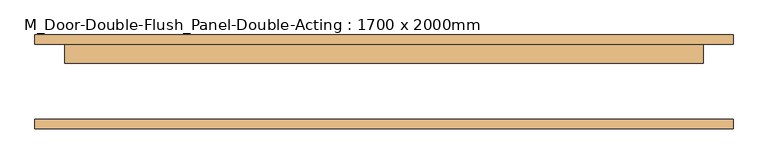
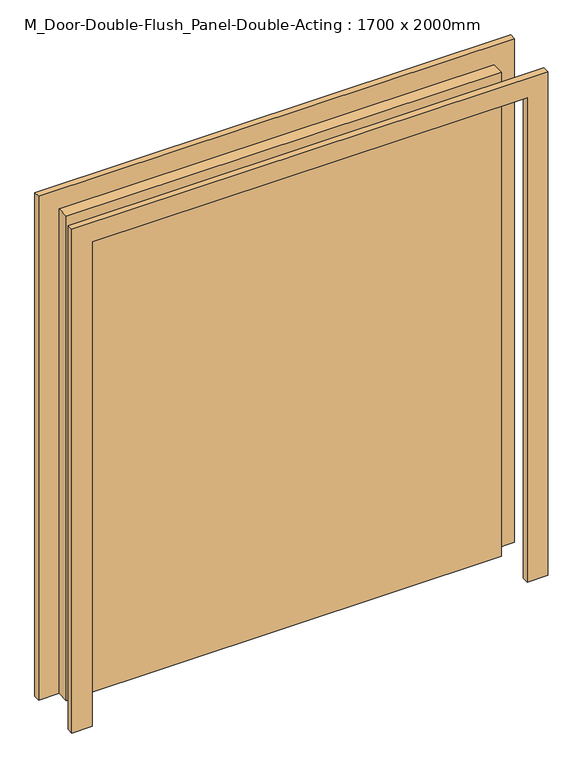
"""IFC4 building model written with IfcOpenShell, lengths in millimetres: door geometry, M_Door-Double-Flush_Panel-Double-Acting : 1700 x 2000mm."""

from ifc_helpers import new_model, si_unit, frame, origin, origin_with_axes, place, context, project, spatial, polyline, outline, extrude, source, transform, mapped, element, save


def m_door_double_flush_panel_double_acting_1700_x_2000mm_0a6d9c7f(model_context):
    return source(origin(), model_context, "Body", "SweptSolid", [
        extrude(outline(polyline([(2080.0, -930.0), (0.0, -930.0), (0.0, -850.0), (2000.0, -850.0), (2000.0, 850.0), (0.0, 850.0), (0.0, 930.0), (2080.0, 930.0), (2080.0, -930.0)])), frame((0.0, 100.0, 0.0), z_axis=(0.0, 1.0, 0.0), x_axis=(0.0, 0.0, 1.0)), (0.0, 0.0, 1.0), 25.0),
        extrude(outline(polyline([(2000.0, -850.0), (2000.0, 850.0), (0.0, 850.0), (0.0, 930.0), (2080.0, 930.0), (2080.0, -930.0), (0.0, -930.0), (0.0, -850.0), (2000.0, -850.0)])), frame((0.0, -125.0, 0.0), z_axis=(0.0, 1.0, 0.0), x_axis=(0.0, 0.0, 1.0)), (0.0, 0.0, 1.0), 25.0),
        extrude(outline(polyline([(-850.0, 100.0), (850.0, 100.0), (850.0, 50.0), (-850.0, 50.0), (-850.0, 100.0)])), origin_with_axes(), (0.0, 0.0, 1.0), 2000.0),
    ])


if __name__ == "__main__":
    model = new_model("IFC4")
    model_context = context("Model", 3, world=origin())
    ifc_project = project(units=[si_unit("LENGTHUNIT", "METRE", prefix="MILLI")], contexts=[model_context])
    site = spatial("IfcSite", under=ifc_project)
    building = spatial("IfcBuilding", under=site)
    placement = place(None, origin())
    m_door_double_flush_panel_double_acting_1700_x_2000mm_shape = m_door_double_flush_panel_double_acting_1700_x_2000mm_0a6d9c7f(model_context)
    element("IfcDoor", 1, ObjectType="M_Door-Double-Flush_Panel-Double-Acting : 1700 x 2000mm", at=placement, inside=building, context=model_context, shape_type="MappedRepresentation", body=[
        mapped(m_door_double_flush_panel_double_acting_1700_x_2000mm_shape, transform((0.0, 0.0, 0.0), x_axis=(1.0, 0.0, 0.0), y_axis=(0.0, 1.0, 0.0), z_axis=(0.0, 0.0, 1.0))),
    ])
    save(model, "model.ifc")

# Revit data of these elements
# Type "M_Door-Double-Flush_Panel-Double-Acting : 1700 x 2000mm"
#   Type Mark = "22"
#   Construction Type Id = "DOOR"
#   Assembly Code = "C1020"
#   Analytic Construction = "Wooden"
#   W = 850 mm
#   Thickness = 50 mm
#   Thermal Resistance (R) = 0.455703 (m²·K)/W
#   Swing Angle [instance default] = 90.00°
#   Heat Transfer Coefficient (U) = 2.19465 W/(m²·K)
#   Height = 2000 mm
#   Trim Projection Ext. = 25 mm
#   Trim Projection Int. = 25 mm
#   Trim Width Ext. = 80 mm
#   Trim Width Int. = 80 mm
#   Width = 1700 mm
#   Define Thermal Properties by = 1
#   Panel Material = Wood - Birch - Solid Stained Light Low Gloss
#   Trim Material = Paint - Sienna
#   Visual Light Transmittance = 0
#   Solar Heat Gain Coefficient = 0
#   Function = (empty or 0)
#   Wall Closure = (empty or 0)
# Element 1 (IfcDoor, "M_Door-Double-Flush_Panel-Double-Acting : 1700 x 2000mm")
#   Materials on its faces: "Paint - Sienna", "Wood - Birch - Solid Stained Light Low Gloss"
# Materials
#   "Wood - Birch - Solid Stained Light Low Gloss": class "Wood", colour RGB 210 159 95, transparency 0, Cost = 0
#   "Paint - Sienna": colour RGB 118 70 51, transparency 0, Cost = 0
